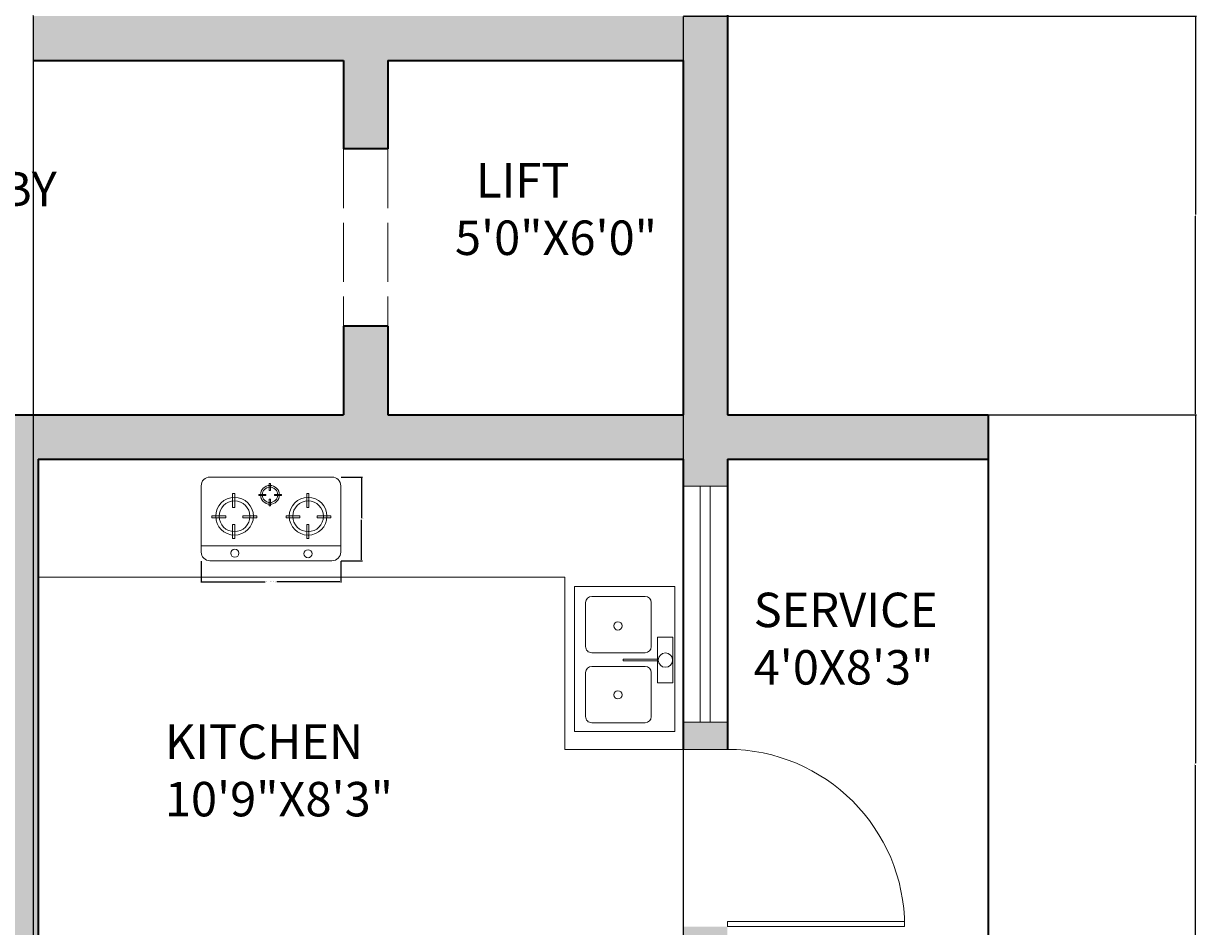
# Model space of a CAD drawing. Units: inches. Extents: x 2540 to 3167, y 3083 to 4007.
# Tile 8 of 15: x 2929 to 3167, y 3359 to 3542. Entities that reach past the tile are written whole.
import ezdxf

# ---------------------------------------------------------------- set-up
doc = ezdxf.new("R2010")
doc.units = ezdxf.units.IN
doc.linetypes.add('ACAD_ISO02W100', pattern=[15, 12, -3])
for name, color, linetype, lineweight in [('A-ANNO-DIMS', 2, 'Continuous', 18), ('A-AREA-IDEN', 7, 'Continuous', 18), ('A-DOOR', 4, 'Continuous', 18), ('A-DOOR-EVTR', 4, 'ACAD_ISO02W100', 18), ('A-EQPM', 9, 'Continuous', 18), ('A-FLOR-CASE', 9, 'Continuous', 18), ('A-FLOR-FIXT', 9, 'Continuous', 18), ('A-FLOR-STRS', 7, 'Continuous', 18), ('A-GLAZ', 4, 'Continuous', 18)]:
    doc.layers.add(name, color=color, linetype=linetype, lineweight=lineweight)
doc.layers.add('A-WALL', color=143, linetype='Continuous', lineweight=35, true_color=0x7aafdf)
doc.layers.add('A-WALL-PATT', color=143, linetype='Continuous', lineweight=13, true_color=0x7aafdf)
doc.styles.get("Standard").update_dxf_attribs({"font": 'arial.ttf'})
doc.dimstyles.get("Standard").update_dxf_attribs({"dimtxt": 0.18, "dimasz": 0.18, "dimexe": 0.18, "dimexo": 0.0625, "dimgap": 0.09, "dimtad": 0, "dimtih": 1, "dimtoh": 1, "dimdec": 4, "dimzin": 0, "dimdsep": 46, "dimtxsty": 'Standard', "dimcen": 0.09, "dimadec": 0, "dimazin": 0, "dimtfac": 1, "dimtdec": 4, "dimtofl": 0, "dimtmove": 0, "dimatfit": 3, "dimfxl": 1, "dimtolj": 1, "dimtzin": 0, "dimarcsym": 0})

# ---------------------------------------------------------------- blocks, each defined once
blk = doc.blocks.new('A$C2A3C6842')
for p, q in [((45, 432), (675, 432)), ((0, 45), (0, 387)), ((351.6, 363.3), (351.6, 398.9)), ((351.6, 398.9), (357.3, 398.9)), ((357.3, 363.3), (351.6, 363.3)), ((357.3, 398.9), (357.3, 363.3)), ((720, 387), (720, 45)), ((161.8, 346.9), (173.2, 346.9)), ((161.8, 275.6), (161.8, 346.9)), ((173.2, 346.9), (173.2, 275.6)), ((298.4, 341.9), (298.4, 336.2)), ((334, 341.9), (298.4, 341.9)), ((298.4, 336.2), (334, 336.2)), ((334, 336.2), (334, 341.9)), ((357.3, 318.8), (351.6, 318.8)), ((351.6, 318.8), (351.6, 283.1)), ((357.3, 283.1), (357.3, 318.8)), ((378.5, 336.2), (378.5, 341.9)), ((378.5, 341.9), (414.2, 341.9)), ((414.2, 336.2), (378.5, 336.2)), ((414.2, 341.9), (414.2, 336.2)), ((544.7, 346.9), (556.1, 346.9)), ((544.7, 275.6), (544.7, 346.9)), ((556.1, 346.9), (556.1, 275.6)), ((173.2, 275.6), (161.8, 275.6)), ((351.6, 283.1), (357.3, 283.1)), ((556.1, 275.6), (544.7, 275.6)), ((55.3, 232.9), (55.3, 221.5)), ((126.6, 232.9), (55.3, 232.9)), ((55.3, 221.5), (126.6, 221.5)), ((126.6, 221.5), (126.6, 232.9)), ((173.2, 186.6), (161.8, 186.6)), ((161.8, 186.6), (161.8, 115.3)), ((173.2, 115.3), (173.2, 186.6)), ((215.6, 221.5), (215.6, 232.9)), ((215.6, 232.9), (286.9, 232.9)), ((286.9, 221.5), (215.6, 221.5)), ((286.9, 232.9), (286.9, 221.5)), ((438.2, 232.9), (438.2, 221.5)), ((509.5, 232.9), (438.2, 232.9)), ((438.2, 221.5), (509.5, 221.5)), ((509.5, 221.5), (509.5, 232.9)), ((556.1, 186.6), (544.7, 186.6)), ((544.7, 186.6), (544.7, 115.3)), ((556.1, 115.3), (556.1, 186.6)), ((598.5, 232.9), (669.8, 232.9)), ((598.5, 221.5), (598.5, 232.9)), ((669.8, 221.5), (598.5, 221.5)), ((669.8, 232.9), (669.8, 221.5)), ((1.2, 76.7), (719.9, 76.7)), ((161.8, 115.3), (173.2, 115.3)), ((544.7, 115.3), (556.1, 115.3)), ((675, 0), (45, 0))]:
    blk.add_line(p, q)
at = {"extrusion": (0, -1e-16, -1)}
for centre, major_axis, start_param, end_param in [((45, 387), (31.8, 31.8), 3.926991, 5.497787), ((172.2, 229.8), (-97.3, 0.1), -0.001099, 6.282086), ((551.8, 229.8), (-97.3, 0.1), -0.001099, 6.282086), ((173.7, 39), (-14.8, 14.8), 5.497787, 11.780972)]:
    blk.add_ellipse(centre, major_axis=major_axis, ratio=1, start_param=start_param, end_param=end_param, dxfattribs=at)
at = {"extrusion": (0, 1e-16, -1)}
blk.add_ellipse((675, 387), major_axis=(-31.8, 31.8), ratio=1, start_param=0.785398, end_param=2.356194, dxfattribs=at)
at = {"extrusion": (-1e-16, -1e-16, -1)}
blk.add_ellipse((355.1, 340.4), major_axis=(48.7, 0.1), ratio=1, start_param=3.144125, end_param=9.42731, dxfattribs=at)
at = {"extrusion": (-1e-16, 0, -1)}
for centre, major_axis, start_param, end_param in [((355.1, 340.4), (-39.7, 0), -0.000334, 6.282851), ((45, 45), (-31.8, 31.8), 3.926991, 5.497787)]:
    blk.add_ellipse(centre, major_axis=major_axis, ratio=1, start_param=start_param, end_param=end_param, dxfattribs=at)
at = {"extrusion": (-1e-16, -4e-16, -1)}
for centre in [(172.2, 229.8), (551.8, 229.8)]:
    blk.add_ellipse(centre, major_axis=(-79.3, 0), ratio=1, start_param=-0.0002116186602152, end_param=6.282973688519371, dxfattribs=at)
at = {"extrusion": (2e-16, -2e-16, -1)}
blk.add_ellipse((551.4, 36.4), major_axis=(14.8, 14.8), ratio=1, start_param=3.926991, end_param=10.210176, dxfattribs=at)
at = {"extrusion": (-2e-16, 1e-16, -1)}
blk.add_ellipse((675, 45), major_axis=(31.8, 31.8), ratio=1, start_param=0.785398, end_param=2.356194, dxfattribs=at)
at = {"text_generation_flag": 4, "flags": 9}
for tag in ['XSIZE', 'YSIZE']:
    blk.add_attdef(tag, (361.3, 264.9), '', height=0.45, rotation=180, dxfattribs=at)
blk = doc.blocks.new('A$C3AD04490')
for p, q in [((0, 640.7), (0, 0)), ((0, 640.7), (924.9, 640.7)), ((614, 627.3), (322.5, 627.3)), ((322.5, 627.3), (322.5, 531.5)), ((614, 531.5), (614, 627.3)), ((924.9, 640.7), (924.9, 0)), ((322.5, 531.5), (614, 531.5)), ((462.6, 311.9), (462.6, 537.2)), ((473.8, 536.8), (473.8, 311.9)), ((62.3, 110.9), (62.3, 451.4)), ((101.4, 490.5), (383.1, 490.5)), ((422.3, 451.4), (422.3, 110.9)), ((508.8, 110.9), (508.8, 451.4)), ((547.9, 490.5), (829.6, 490.5)), ((868.8, 451.4), (868.8, 110.9)), ((463.4, 310.9), (474.3, 310.9)), ((383.1, 71.7), (101.4, 71.7)), ((829.6, 71.7), (547.9, 71.7)), ((924.9, 0), (0, 0))]:
    blk.add_line(p, q)
for centre, radius in [((469, 581.2), 45.9), ((250.7, 278.1), 26.4), ((690.5, 278.1), 26.4)]:
    blk.add_circle(centre, radius)
for centre, start, end in [((101.4, 451.4), 90, 180), ((383.1, 451.4), 0, 90), ((547.9, 451.4), 90, 180), ((829.6, 451.4), 0, 90), ((101.4, 110.9), 180, 270), ((383.1, 110.9), 270, 0), ((547.9, 110.9), 180, 270), ((829.6, 110.9), 270, 0)]:
    blk.add_arc(centre, 39.1, start, end)
blk = doc.blocks.new('DOOR-SWING-36IN')
for p, q in [((36, 0), (0, 0)), ((36, 1), (0.01, 1)), ((36, 1), (36, 0))]:
    blk.add_line(p, q)
blk.add_arc((36, 0), 36, 90, 180)
blk = doc.blocks.new('WIN-48IN')
for p, q in [((0, 48), (9, 48)), ((3.5, 0), (3.5, 48)), ((5.5, 0), (5.5, 48)), ((0, 0), (9, 0))]:
    blk.add_line(p, q)
blk = doc.blocks.new('*D33')
at = {"layer": 'A-ANNO-DIMS', "color": 0, "lineweight": -2, "transparency": 16777216}
for p, q in [((2964.61, 3432.97), (2964.61, 3428.6)), ((2992.96, 3432.97), (2992.96, 3428.6)), ((2964.79, 3428.78), (2977.6, 3428.78)), ((2992.78, 3428.78), (2979.98, 3428.78))]:
    blk.add_line(p, q, dxfattribs=at)
at = {"layer": 'A-ANNO-DIMS', "color": 0, "transparency": 16777216}
for points in [[(2964.79, 3428.81), (2964.79, 3428.75), (2964.61, 3428.78)], [(2992.78, 3428.81), (2992.78, 3428.75), (2992.96, 3428.78)]]:
    blk.add_solid(points, dxfattribs=at)
at = {"layer": 'Defpoints', "color": 0, "transparency": 16777216}
for p in [(2964.61, 3433.03), (2992.96, 3433.03), (2992.96, 3428.78)]:
    blk.add_point(p, dxfattribs=at)
at = {"layer": 'A-ANNO-DIMS', "color": 0, "transparency": 16777216, "insert": (2978.79, 3428.78), "char_height": 0.18, "attachment_point": 5}
blk.add_mtext('\\A1;COOKTOP 28 TYP.', dxfattribs=at)
blk = doc.blocks.new('*D34')
at = {"layer": 'A-ANNO-DIMS', "color": 0, "lineweight": -2, "transparency": 16777216}
for p, q in [((2993.02, 3450.04), (2997.39, 3450.04)), ((2997.21, 3449.86), (2997.21, 3441.71)), ((2997.21, 3433.21), (2997.21, 3441.35)), ((2993.02, 3433.03), (2997.39, 3433.03))]:
    blk.add_line(p, q, dxfattribs=at)
at = {"layer": 'A-ANNO-DIMS', "color": 0, "transparency": 16777216}
for points in [[(2997.18, 3449.86), (2997.24, 3449.86), (2997.21, 3450.04)], [(2997.18, 3433.21), (2997.24, 3433.21), (2997.21, 3433.03)]]:
    blk.add_solid(points, dxfattribs=at)
at = {"layer": 'Defpoints', "color": 0, "transparency": 16777216}
for p in [(2992.96, 3450.04), (2997.21, 3450.04), (2992.96, 3433.03)]:
    blk.add_point(p, dxfattribs=at)
at = {"layer": 'A-ANNO-DIMS', "color": 0, "transparency": 16777216, "insert": (2997.21, 3441.53), "char_height": 0.18, "attachment_point": 5}
blk.add_mtext('\\A1;17 TYP.', dxfattribs=at)
blk = doc.blocks.new('*D51')
at = {"layer": 'A-ANNO-DIMS', "color": 0, "lineweight": -2, "transparency": 16777216}
for p, q in [((3062.57, 3543.71), (3166.79, 3543.71)), ((3166.61, 3543.53), (3166.61, 3503.4)), ((3166.61, 3462.89), (3166.61, 3503.03)), ((3124.57, 3462.71), (3166.79, 3462.71))]:
    blk.add_line(p, q, dxfattribs=at)
at = {"layer": 'A-ANNO-DIMS', "color": 0, "transparency": 16777216}
for points in [[(3166.58, 3543.53), (3166.64, 3543.53), (3166.61, 3543.71)], [(3166.58, 3462.89), (3166.64, 3462.89), (3166.61, 3462.71)]]:
    blk.add_solid(points, dxfattribs=at)
at = {"layer": 'Defpoints', "color": 0, "transparency": 16777216}
for p in [(3062.51, 3543.71), (3124.51, 3462.71), (3166.61, 3462.71)]:
    blk.add_point(p, dxfattribs=at)
at = {"layer": 'A-ANNO-DIMS', "color": 0, "transparency": 16777216, "insert": (3166.61, 3503.21), "char_height": 0.18, "attachment_point": 5}
blk.add_mtext('\\A1;81', dxfattribs=at)
blk = doc.blocks.new('*D52')
at = {"layer": 'A-ANNO-DIMS', "color": 0, "lineweight": -2, "transparency": 16777216}
for p, q in [((3124.57, 3462.71), (3166.79, 3462.71)), ((3166.61, 3462.53), (3166.61, 3391.89)), ((3166.61, 3320.89), (3166.61, 3391.53)), ((3124.57, 3320.71), (3166.79, 3320.71))]:
    blk.add_line(p, q, dxfattribs=at)
at = {"layer": 'A-ANNO-DIMS', "color": 0, "transparency": 16777216}
for points in [[(3166.58, 3462.53), (3166.64, 3462.53), (3166.61, 3462.71)], [(3166.58, 3320.89), (3166.64, 3320.89), (3166.61, 3320.71)]]:
    blk.add_solid(points, dxfattribs=at)
at = {"layer": 'Defpoints', "color": 0, "transparency": 16777216}
for p in [(3124.51, 3462.71), (3124.51, 3320.71), (3166.61, 3320.71)]:
    blk.add_point(p, dxfattribs=at)
at = {"layer": 'A-ANNO-DIMS', "color": 0, "transparency": 16777216, "insert": (3166.61, 3391.71), "char_height": 0.18, "attachment_point": 5}
blk.add_mtext('\\A1;142', dxfattribs=at)
blk = doc.blocks.new('*D54')
at = {"layer": 'A-ANNO-DIMS', "color": 0, "lineweight": -2, "transparency": 16777216}
for p, q in [((2930.51, 3543.65), (2930.51, 3083.43)), ((3062.51, 3543.65), (3062.51, 3083.43)), ((2930.69, 3083.61), (2996.23, 3083.61)), ((3062.33, 3083.61), (2996.79, 3083.61))]:
    blk.add_line(p, q, dxfattribs=at)
at = {"layer": 'A-ANNO-DIMS', "color": 0, "transparency": 16777216}
for points in [[(2930.69, 3083.64), (2930.69, 3083.58), (2930.51, 3083.61)], [(3062.33, 3083.64), (3062.33, 3083.58), (3062.51, 3083.61)]]:
    blk.add_solid(points, dxfattribs=at)
at = {"layer": 'Defpoints', "color": 0, "transparency": 16777216}
for p in [(2930.51, 3543.71), (3062.51, 3543.71), (3062.51, 3083.61)]:
    blk.add_point(p, dxfattribs=at)
at = {"layer": 'A-ANNO-DIMS', "color": 0, "transparency": 16777216, "insert": (2996.51, 3083.61), "char_height": 0.18, "attachment_point": 5}
blk.add_mtext('\\A1;132', dxfattribs=at)
blk = doc.blocks.new('*D55')
at = {"layer": 'A-ANNO-DIMS', "color": 0, "lineweight": -2, "transparency": 16777216}
for p, q in [((2868.51, 3564.65), (2868.51, 3083.43)), ((2930.51, 3543.65), (2930.51, 3083.43)), ((2868.69, 3083.61), (2899.29, 3083.61)), ((2930.33, 3083.61), (2899.73, 3083.61))]:
    blk.add_line(p, q, dxfattribs=at)
at = {"layer": 'A-ANNO-DIMS', "color": 0, "transparency": 16777216}
for points in [[(2868.69, 3083.64), (2868.69, 3083.58), (2868.51, 3083.61)], [(2930.33, 3083.64), (2930.33, 3083.58), (2930.51, 3083.61)]]:
    blk.add_solid(points, dxfattribs=at)
at = {"layer": 'Defpoints', "color": 0, "transparency": 16777216}
for p in [(2868.51, 3564.71), (2930.51, 3543.71), (2930.51, 3083.61)]:
    blk.add_point(p, dxfattribs=at)
at = {"layer": 'A-ANNO-DIMS', "color": 0, "transparency": 16777216, "insert": (2899.51, 3083.61), "char_height": 0.18, "attachment_point": 5}
blk.add_mtext('\\A1;62', dxfattribs=at)

msp = doc.modelspace()

# ---------------------------------------------------------------- hatches: boundary and pattern name
at = {"layer": 'A-WALL-PATT'}
h = msp.add_hatch(color=256, dxfattribs=at)
h.dxf.hatch_style = 1
h.paths.add_polyline_path([(2805.51, 3803.71), (2800.51, 3803.71), (2800.51, 3799.71), (2621.51, 3799.71), (2621.51, 3823.71), (2612.51, 3823.71), (2612.51, 3794.71), (2636.51, 3794.71), (2636.51, 3782.71), (2645.51, 3782.71), (2645.51, 3794.71), (2805.51, 3794.71)])
h.paths.add_polyline_path([(2810.51, 3564.71), (2868.51, 3564.71), (2868.51, 3627.71), (2872.51, 3627.71), (2872.51, 3636.71), (2864.51, 3636.71), (2864.51, 3674.71), (2797.51, 3674.71), (2797.51, 3669.71), (2801.51, 3669.71), (2801.51, 3628.63), (2806.51, 3628.63), (2806.51, 3669.71), (2859.51, 3669.71), (2859.51, 3573.71), (2806.51, 3573.71), (2806.51, 3598.63), (2801.51, 3598.63), (2801.51, 3549.71), (2645.51, 3549.71), (2645.51, 3573.71), (2636.51, 3573.71), (2636.51, 3516.71), (2645.51, 3516.71), (2645.51, 3540.71), (2801.51, 3540.71), (2801.51, 3504.71), (2801.51, 3500.71), (2806.51, 3500.71), (2806.51, 3504.71), (2859.51, 3504.71), (2859.51, 3420.71), (2806.51, 3420.71), (2806.51, 3470.71), (2801.51, 3470.71), (2801.51, 3420.71), (2797.51, 3420.71), (2797.51, 3415.71), (2864.51, 3415.71), (2864.51, 3453.71), (2868.51, 3453.71), (2868.51, 3513.71), (2810.51, 3513.71)])
h.paths.add_polyline_path([(2645.51, 3415.71), (2761.51, 3415.71), (2761.51, 3420.71), (2645.51, 3420.71), (2645.51, 3444.71), (2636.51, 3444.71), (2636.51, 3403.71), (2645.51, 3403.71)])
h.paths.add_polyline_path([(2645.51, 3307.71), (2636.51, 3307.71), (2636.51, 3295.71), (2612.51, 3295.71), (2612.51, 3149.71), (2645.51, 3149.71), (2645.51, 3158.71), (2621.51, 3158.71), (2621.51, 3290.71), (2801.51, 3290.71), (2801.51, 3286.71), (2806.51, 3286.71), (2806.51, 3295.71), (2645.51, 3295.71)])
h.paths.add_polyline_path([(2762.01, 3158.71), (2746.51, 3158.71), (2746.51, 3240.71), (2750.51, 3240.71), (2750.51, 3245.71), (2741.51, 3245.71), (2741.51, 3158.71), (2717.51, 3158.71), (2717.51, 3149.71), (2762.01, 3149.71)], flags=17)
h.paths.add_polyline_path([(2810.51, 3173.71), (2822.51, 3173.71), (2822.51, 3182.71), (2806.51, 3182.71), (2806.51, 3250.71), (2801.51, 3250.71), (2801.51, 3245.71), (2780.51, 3245.71), (2780.51, 3240.71), (2801.51, 3240.71), (2801.51, 3158.71), (2786.01, 3158.71), (2786.01, 3149.71), (2810.51, 3149.71)])
h.paths.add_polyline_path([(2931.51, 3290.71), (2935.51, 3290.71), (2935.51, 3295.71), (2926.51, 3295.71), (2926.51, 3182.71), (2910.51, 3182.71), (2910.51, 3173.71), (2922.51, 3173.71), (2922.51, 3149.71), (2987.51, 3149.71), (2987.51, 3158.71), (2931.51, 3158.71)])
h.paths.add_polyline_path([(3124.51, 3295.71), (3086.51, 3295.71), (3018.51, 3295.71), (3018.51, 3290.71), (3115.51, 3290.71), (3115.51, 3158.71), (3059.51, 3158.71), (3059.51, 3149.71), (3124.51, 3149.71)])
h.paths.add_polyline_path([(2988.51, 3295.71), (2984.51, 3295.71), (2984.51, 3349.71), (3086.51, 3349.71), (3086.51, 3320.71), (3124.51, 3320.71), (3124.51, 3354.71), (3071.51, 3354.71), (3071.51, 3358.71), (3062.51, 3358.71), (3062.51, 3354.71), (2979.51, 3354.71), (2979.51, 3295.71), (2971.51, 3295.71), (2971.51, 3290.71), (2988.51, 3290.71)])
h.paths.add_polyline_path([(3095.51, 3325.71), (3095.51, 3349.71), (3119.51, 3349.71), (3119.51, 3325.71)], flags=16)
h.paths.add_polyline_path([(3124.51, 3462.71), (3071.51, 3462.71), (3071.51, 3627.71), (3124.51, 3627.71), (3124.51, 3693.71), (3095.51, 3693.71), (3095.51, 3702.71), (3086.51, 3702.71), (3086.51, 3684.71), (3086.51, 3636.71), (2930.51, 3636.71), (2930.51, 3768.71), (2934.51, 3768.71), (2934.51, 3773.71), (2930.51, 3773.71), (2925.51, 3773.71), (2925.51, 3730.71), (2864.51, 3730.71), (2864.51, 3760.71), (2859.51, 3760.71), (2859.51, 3725.71), (2925.51, 3725.71), (2925.51, 3636.71), (2908.51, 3636.71), (2908.51, 3627.71), (3062.51, 3627.71), (3062.51, 3543.71), (2930.51, 3543.71), (2930.51, 3534.71), (2993.51, 3534.71), (2993.51, 3516.71), (3002.51, 3516.71), (3002.51, 3534.71), (3062.51, 3534.71), (3062.51, 3462.71), (3002.51, 3462.71), (3002.51, 3480.71), (2993.51, 3480.71), (2993.51, 3462.71), (2916.51, 3462.71), (2916.51, 3453.71), (2926.51, 3453.71), (2926.51, 3361.71), (2859.51, 3361.71), (2859.51, 3338.71), (2864.51, 3338.71), (2864.51, 3356.71), (2926.51, 3356.71), (2926.51, 3338.71), (2931.51, 3338.71), (2931.51, 3453.71), (3062.51, 3453.71), (3062.51, 3448.21), (3071.51, 3448.21), (3071.51, 3453.71), (3124.51, 3453.71)])
h = msp.add_hatch(color=256, dxfattribs=at)
h.dxf.hatch_style = 1
h.paths.add_polyline_path([(3071.51, 3400.21), (3062.51, 3400.21), (3062.51, 3394.71), (3071.51, 3394.71)])

# ---------------------------------------------------------------- linework, layer by layer
at = {"layer": 'A-DOOR-EVTR'}
for p, q in [((2993.51, 3516.71), (2993.51, 3480.71)), ((3002.51, 3516.71), (3002.51, 3480.71))]:
    msp.add_line(p, q, dxfattribs=at)
at = {"layer": 'A-FLOR-CASE'}
for p, q in [((2931.51, 3429.71), (3038.51, 3429.71)), ((3038.51, 3429.71), (3038.51, 3394.71)), ((3038.51, 3394.71), (3071.51, 3394.71))]:
    msp.add_line(p, q, dxfattribs=at)
at = {"layer": 'A-FLOR-STRS'}
msp.add_line((2930.51, 3627.71), (2930.51, 3534.71), dxfattribs=at)
at = {"layer": 'A-WALL'}
for p, q in [((3071.51, 3627.71), (3071.51, 3462.71)), ((2930.51, 3534.71), (2993.51, 3534.71)), ((2993.51, 3534.71), (2993.51, 3516.71)), ((3002.51, 3534.71), (3002.51, 3516.71)), ((3002.51, 3534.71), (3062.51, 3534.71)), ((3062.51, 3534.71), (3062.51, 3462.71)), ((3002.51, 3516.71), (2993.51, 3516.71)), ((3002.51, 3480.71), (2993.51, 3480.71)), ((2993.51, 3480.71), (2993.51, 3462.71)), ((3002.51, 3480.71), (3002.51, 3462.71)), ((2916.51, 3462.71), (2993.51, 3462.71)), ((3002.51, 3462.71), (3062.51, 3462.71)), ((3071.51, 3462.71), (3124.51, 3462.71)), ((3124.51, 3462.71), (3124.51, 3320.71)), ((2931.51, 3453.71), (2931.51, 3338.71)), ((2931.51, 3453.71), (3062.51, 3453.71)), ((3062.51, 3453.71), (3062.51, 3394.71)), ((3071.51, 3453.71), (3071.51, 3394.71)), ((3071.51, 3453.71), (3124.51, 3453.71))]:
    msp.add_line(p, q, dxfattribs=at)

# ---------------------------------------------------------------- block references
at = {"layer": 'A-DOOR', "extrusion": (0, 0, -1), "zscale": -1}
msp.add_blockref('DOOR-SWING-36IN', (-3107.51, 3358.71), dxfattribs=at)
at = {"layer": 'A-EQPM', "xscale": 0.0393700787401575, "yscale": 0.0393700787401575, "zscale": 0.0393700787401575}
msp.add_blockref('A$C2A3C6842', (2964.61, 3433.03), dxfattribs=at)
at = {"layer": 'A-FLOR-FIXT', "xscale": 0.0318479740928733, "yscale": 0.0318479740928733, "zscale": 0.0318479740928733, "rotation": 270}
msp.add_blockref('A$C3AD04490', (3040.42, 3427.79), dxfattribs=at)
at = {"layer": 'A-GLAZ'}
msp.add_blockref('WIN-48IN', (3062.51, 3400.21), dxfattribs=at)

# ---------------------------------------------------------------- texts
at = {"layer": 'A-AREA-IDEN', "char_height": 7, "attachment_point": 1}
for s, width, insert in [('  LIFT\\P5\'0"X6\'0"', 34.4573, (3016.17, 3513.84)), ('LOBBY', 34.4573, (2905.37, 3512.07)), ('SERVICE\\P4\'0X8\'3"', 37.9387, (3076.85, 3426.55)), ('KITCHEN\\P10\'9"X8\'3"', 74.1323, (2957.24, 3399.77))]:
    msp.add_mtext_dynamic_manual_height_columns(s, width=width, gutter_width=12.5, heights=[0], dxfattribs=dict(at, insert=insert))

# ---------------------------------------------------------------- dimensions: what is measured, and where the dimension line sits
at = {"layer": 'A-ANNO-DIMS'}
for base, p1, p2, picture, middle in [((2930.51, 3083.61), (2868.51, 3564.71), (2930.51, 3543.71), '*D55', (2899.51, 3083.61)), ((3062.51, 3083.61), (2930.51, 3543.71), (3062.51, 3543.71), '*D54', (2996.51, 3083.61))]:
    dim = msp.add_linear_dim(base=base, p1=p1, p2=p2, dimstyle='Standard', override={"dimdec": 0, "dimlfac": 1, "dimrnd": 0, "dimzin": 0, "dimdsep": 46, "dimlunit": 2}, dxfattribs=at)
    dim.commit()
    dim.dimension.update_dxf_attribs({"geometry": picture, "text_midpoint": middle})
for base, p1, p2, picture, middle in [((3166.61, 3462.71), (3062.51, 3543.71), (3124.51, 3462.71), '*D51', (3166.61, 3503.21)), ((3166.61, 3320.71), (3124.51, 3462.71), (3124.51, 3320.71), '*D52', (3166.61, 3391.71))]:
    dim = msp.add_linear_dim(base=base, p1=p1, p2=p2, angle=90, dimstyle='Standard', override={"dimdec": 0, "dimlfac": 1, "dimrnd": 0, "dimzin": 0, "dimdsep": 46, "dimlunit": 2}, dxfattribs=at)
    dim.commit()
    dim.dimension.update_dxf_attribs({"geometry": picture, "text_midpoint": middle})
dim = msp.add_linear_dim(base=(2997.21, 3450.04), p1=(2992.96, 3433.03), p2=(2992.96, 3450.04), angle=90, text='<> TYP.', dimstyle='Standard', override={"dimdec": 0, "dimlfac": 1, "dimrnd": 0, "dimzin": 0, "dimdsep": 46, "dimlunit": 2}, dxfattribs=at)
dim.commit()
dim.dimension.update_dxf_attribs({"geometry": '*D34', "text_midpoint": (2997.21, 3441.53)})
dim = msp.add_linear_dim(base=(2992.96, 3428.78), p1=(2964.61, 3433.03), p2=(2992.96, 3433.03), text='COOKTOP <> TYP.', dimstyle='Standard', override={"dimdec": 0, "dimlfac": 1, "dimrnd": 0, "dimzin": 0, "dimdsep": 46, "dimlunit": 2}, dxfattribs=at)
dim.commit()
dim.dimension.update_dxf_attribs({"geometry": '*D33', "text_midpoint": (2978.79, 3428.78)})

doc.saveas('drawing.dxf')
